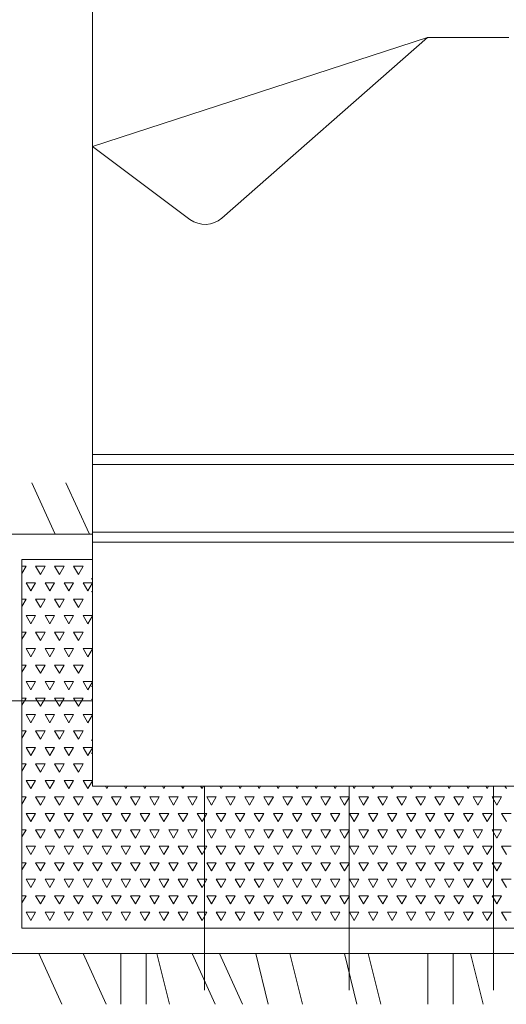
# Model space of a CAD drawing. Units: millimetres. Extents: x 225995 to 227247, y 225507 to 226008.
# Tile 6 of 23: x 226421 to 226461, y 225786 to 225867. Entities that reach past the tile are written whole.
import ezdxf

# ---------------------------------------------------------------- set-up
doc = ezdxf.new("R2010")
doc.units = ezdxf.units.MM
doc.layers.add('A-FLOR-PATT', color=8, linetype='Continuous', lineweight=13)
doc.layers.add('A-FURN', color=9, linetype='Continuous', lineweight=18)

# ---------------------------------------------------------------- blocks, each defined once
blk = doc.blocks.new('A$C6D2A2628')
for p, q in [((0.291, 0.4297), (0.291, 2.4297)), ((0.291, 1.6908), (0.9515, 1.9058)), ((0.9515, 1.9058), (0.5462, 1.5497)), ((0.9515, 1.9058), (1.1116, 1.9058)), ((0.4832, 1.5472), (0.291, 1.6908)), ((0.291, 1.0837), (1.791, 1.0837)), ((0.291, 1.0637), (1.791, 1.0637)), ((0.1716, 1.0278), (0.217, 0.9278)), ((0.2388, 1.0278), (0.2843, 0.9278)), ((0.291, 0.9267), (0.1019, 0.9267)), ((0.291, 0.9307), (1.791, 0.9307)), ((0.291, 0.9107), (1.791, 0.9107)), ((0.291, 0.8767), (0.1519, 0.8767)), ((0.1519, 0.8767), (0.1519, 0.15)), ((0.1519, 0.8494), (0.1601, 0.8636)), ((0.1519, 0.8636), (0.1601, 0.8636)), ((0.1882, 0.8473), (0.1788, 0.8636)), ((0.1788, 0.8636), (0.1976, 0.8636)), ((0.1882, 0.8473), (0.1976, 0.8636)), ((0.2257, 0.8473), (0.2163, 0.8636)), ((0.2163, 0.8636), (0.2351, 0.8636)), ((0.2257, 0.8473), (0.2351, 0.8636)), ((0.2632, 0.8473), (0.2538, 0.8636)), ((0.2538, 0.8636), (0.2726, 0.8636)), ((0.2632, 0.8473), (0.2726, 0.8636)), ((0.291, 0.8376), (0.2893, 0.8393)), ((0.1695, 0.8148), (0.1601, 0.8311)), ((0.1601, 0.8311), (0.1788, 0.8311)), ((0.1695, 0.8148), (0.1788, 0.8311)), ((0.207, 0.8148), (0.1976, 0.8311)), ((0.1976, 0.8311), (0.2163, 0.8311)), ((0.207, 0.8148), (0.2163, 0.8311)), ((0.2445, 0.8148), (0.2351, 0.8311)), ((0.2351, 0.8311), (0.2538, 0.8311)), ((0.2445, 0.8148), (0.2538, 0.8311)), ((0.282, 0.8148), (0.2726, 0.8311)), ((0.2726, 0.8311), (0.291, 0.8311)), ((0.282, 0.8148), (0.291, 0.8305)), ((0.1519, 0.7844), (0.1601, 0.7986)), ((0.1519, 0.7986), (0.1601, 0.7986)), ((0.1882, 0.7824), (0.1788, 0.7986)), ((0.1788, 0.7986), (0.1976, 0.7986)), ((0.1882, 0.7824), (0.1976, 0.7986)), ((0.2257, 0.7824), (0.2163, 0.7986)), ((0.2163, 0.7986), (0.2351, 0.7986)), ((0.2257, 0.7824), (0.2351, 0.7986)), ((0.2632, 0.7824), (0.2538, 0.7986)), ((0.2538, 0.7986), (0.2726, 0.7986)), ((0.2632, 0.7824), (0.2726, 0.7986)), ((0.291, 0.8144), (0.2893, 0.8128)), ((0.1695, 0.7499), (0.1601, 0.7661)), ((0.1601, 0.7661), (0.1788, 0.7661)), ((0.1695, 0.7499), (0.1788, 0.7661)), ((0.207, 0.7499), (0.1976, 0.7661)), ((0.1976, 0.7661), (0.2163, 0.7661)), ((0.207, 0.7499), (0.2163, 0.7661)), ((0.2445, 0.7499), (0.2351, 0.7661)), ((0.2351, 0.7661), (0.2538, 0.7661)), ((0.2445, 0.7499), (0.2538, 0.7661)), ((0.282, 0.7499), (0.2726, 0.7661)), ((0.2726, 0.7661), (0.291, 0.7661)), ((0.282, 0.7499), (0.291, 0.7655)), ((0.1519, 0.7195), (0.1601, 0.7337)), ((0.1519, 0.7337), (0.1601, 0.7337)), ((0.1882, 0.7174), (0.1788, 0.7337)), ((0.1788, 0.7337), (0.1976, 0.7337)), ((0.1882, 0.7174), (0.1976, 0.7337)), ((0.2257, 0.7174), (0.2163, 0.7337)), ((0.2163, 0.7337), (0.2351, 0.7337)), ((0.2257, 0.7174), (0.2351, 0.7337)), ((0.2632, 0.7174), (0.2538, 0.7337)), ((0.2538, 0.7337), (0.2726, 0.7337)), ((0.2632, 0.7174), (0.2726, 0.7337)), ((0.1695, 0.6849), (0.1601, 0.7012)), ((0.1601, 0.7012), (0.1788, 0.7012)), ((0.1695, 0.6849), (0.1788, 0.7012)), ((0.207, 0.6849), (0.1976, 0.7012)), ((0.1976, 0.7012), (0.2163, 0.7012)), ((0.207, 0.6849), (0.2163, 0.7012)), ((0.2445, 0.6849), (0.2351, 0.7012)), ((0.2351, 0.7012), (0.2538, 0.7012)), ((0.2445, 0.6849), (0.2538, 0.7012)), ((0.282, 0.6849), (0.2726, 0.7012)), ((0.2726, 0.7012), (0.291, 0.7012)), ((0.282, 0.6849), (0.291, 0.7006)), ((0.1519, 0.6545), (0.1601, 0.6687)), ((0.1519, 0.6687), (0.1601, 0.6687)), ((0.1882, 0.6525), (0.1788, 0.6687)), ((0.1788, 0.6687), (0.1976, 0.6687)), ((0.1882, 0.6525), (0.1976, 0.6687)), ((0.2257, 0.6525), (0.2163, 0.6687)), ((0.2163, 0.6687), (0.2351, 0.6687)), ((0.2257, 0.6525), (0.2351, 0.6687)), ((0.2632, 0.6525), (0.2538, 0.6687)), ((0.2538, 0.6687), (0.2726, 0.6687)), ((0.2632, 0.6525), (0.2726, 0.6687)), ((0.1695, 0.62), (0.1601, 0.6362)), ((0.1601, 0.6362), (0.1788, 0.6362)), ((0.1695, 0.62), (0.1788, 0.6362)), ((0.207, 0.62), (0.1976, 0.6362)), ((0.1976, 0.6362), (0.2163, 0.6362)), ((0.207, 0.62), (0.2163, 0.6362)), ((0.2445, 0.62), (0.2351, 0.6362)), ((0.2351, 0.6362), (0.2538, 0.6362)), ((0.2445, 0.62), (0.2538, 0.6362)), ((0.282, 0.62), (0.2726, 0.6362)), ((0.2726, 0.6362), (0.291, 0.6362)), ((0.282, 0.62), (0.291, 0.6356)), ((0.291, 0.6255), (0.2893, 0.6271)), ((0.1519, 0.5896), (0.1601, 0.6037)), ((0.1519, 0.6037), (0.1601, 0.6037)), ((0.1882, 0.5875), (0.1788, 0.6037)), ((0.1788, 0.6037), (0.1976, 0.6037)), ((0.1882, 0.5875), (0.1976, 0.6037)), ((0.2257, 0.5875), (0.2163, 0.6037)), ((0.2163, 0.6037), (0.2351, 0.6037)), ((0.2257, 0.5875), (0.2351, 0.6037)), ((0.2632, 0.5875), (0.2538, 0.6037)), ((0.2538, 0.6037), (0.2726, 0.6037)), ((0.2632, 0.5875), (0.2726, 0.6037)), ((0.291, 0.6023), (0.2893, 0.6006)), ((0.1695, 0.555), (0.1601, 0.5713)), ((0.1601, 0.5713), (0.1788, 0.5713)), ((0.1695, 0.555), (0.1788, 0.5713)), ((0.207, 0.555), (0.1976, 0.5713)), ((0.1976, 0.5713), (0.2163, 0.5713)), ((0.207, 0.555), (0.2163, 0.5713)), ((0.2445, 0.555), (0.2351, 0.5713)), ((0.2351, 0.5713), (0.2538, 0.5713)), ((0.2445, 0.555), (0.2538, 0.5713)), ((0.282, 0.555), (0.2726, 0.5713)), ((0.2726, 0.5713), (0.291, 0.5713)), ((0.282, 0.555), (0.291, 0.5707)), ((0.1519, 0.5246), (0.1601, 0.5388)), ((0.1519, 0.5388), (0.1601, 0.5388)), ((0.1882, 0.5226), (0.1788, 0.5388)), ((0.1788, 0.5388), (0.1976, 0.5388)), ((0.1882, 0.5226), (0.1976, 0.5388)), ((0.2257, 0.5226), (0.2163, 0.5388)), ((0.2163, 0.5388), (0.2351, 0.5388)), ((0.2257, 0.5226), (0.2351, 0.5388)), ((0.2632, 0.5226), (0.2538, 0.5388)), ((0.2538, 0.5388), (0.2726, 0.5388)), ((0.2632, 0.5226), (0.2726, 0.5388)), ((0.1695, 0.4901), (0.1601, 0.5063)), ((0.1601, 0.5063), (0.1788, 0.5063)), ((0.1695, 0.4901), (0.1788, 0.5063)), ((0.207, 0.4901), (0.1976, 0.5063)), ((0.1976, 0.5063), (0.2163, 0.5063)), ((0.207, 0.4901), (0.2163, 0.5063)), ((0.2445, 0.4901), (0.2351, 0.5063)), ((0.2351, 0.5063), (0.2538, 0.5063)), ((0.2445, 0.4901), (0.2538, 0.5063)), ((0.282, 0.4901), (0.2726, 0.5063)), ((0.2726, 0.5063), (0.291, 0.5063)), ((0.282, 0.4901), (0.291, 0.5057)), ((0.291, 0.5194), (0.2893, 0.5211)), ((0.291, 0.4962), (0.2893, 0.4946)), ((0.1519, 0.4597), (0.1601, 0.4738)), ((0.1519, 0.4738), (0.1601, 0.4738)), ((0.1882, 0.4576), (0.1788, 0.4738)), ((0.1788, 0.4738), (0.1976, 0.4738)), ((0.1882, 0.4576), (0.1976, 0.4738)), ((0.2257, 0.4576), (0.2163, 0.4738)), ((0.2163, 0.4738), (0.2351, 0.4738)), ((0.2257, 0.4576), (0.2351, 0.4738)), ((0.2632, 0.4576), (0.2538, 0.4738)), ((0.2538, 0.4738), (0.2726, 0.4738)), ((0.2632, 0.4576), (0.2726, 0.4738)), ((0.1695, 0.4251), (0.1601, 0.4414)), ((0.1601, 0.4414), (0.1788, 0.4414)), ((0.1695, 0.4251), (0.1788, 0.4414)), ((0.207, 0.4251), (0.1976, 0.4414)), ((0.1976, 0.4414), (0.2163, 0.4414)), ((0.207, 0.4251), (0.2163, 0.4414)), ((0.2445, 0.4251), (0.2351, 0.4414)), ((0.2351, 0.4414), (0.2538, 0.4414)), ((0.2445, 0.4251), (0.2538, 0.4414)), ((0.282, 0.4251), (0.2726, 0.4414)), ((0.2726, 0.4414), (0.291, 0.4414)), ((0.282, 0.4251), (0.291, 0.4408)), ((1.791, 0.4297), (0.291, 0.4297)), ((0.3195, 0.4251), (0.3168, 0.4297)), ((0.3195, 0.4251), (0.3221, 0.4297)), ((0.357, 0.4251), (0.3543, 0.4297)), ((0.357, 0.4251), (0.3596, 0.4297)), ((0.3945, 0.4251), (0.3918, 0.4297)), ((0.3945, 0.4251), (0.3971, 0.4297)), ((0.432, 0.4251), (0.4293, 0.4297)), ((0.432, 0.4251), (0.4346, 0.4297)), ((0.4695, 0.4251), (0.4668, 0.4297)), ((0.4695, 0.4251), (0.4721, 0.4297)), ((0.507, 0.4251), (0.5043, 0.4297)), ((0.507, 0.4251), (0.5096, 0.4297)), ((0.5445, 0.4251), (0.5418, 0.4297)), ((0.5445, 0.4251), (0.5471, 0.4297)), ((0.582, 0.4251), (0.5793, 0.4297)), ((0.582, 0.4251), (0.5846, 0.4297)), ((0.6195, 0.4251), (0.6168, 0.4297)), ((0.6195, 0.4251), (0.6221, 0.4297)), ((0.657, 0.4251), (0.6543, 0.4297)), ((0.657, 0.4251), (0.6596, 0.4297)), ((0.6945, 0.4251), (0.6918, 0.4297)), ((0.6945, 0.4251), (0.6971, 0.4297)), ((0.732, 0.4251), (0.7293, 0.4297)), ((0.732, 0.4251), (0.7346, 0.4297)), ((0.7695, 0.4251), (0.7668, 0.4297)), ((0.7695, 0.4251), (0.7721, 0.4297)), ((0.807, 0.4251), (0.8043, 0.4297)), ((0.807, 0.4251), (0.8096, 0.4297)), ((0.8445, 0.4251), (0.8418, 0.4297)), ((0.8445, 0.4251), (0.8471, 0.4297)), ((0.882, 0.4251), (0.8793, 0.4297)), ((0.882, 0.4251), (0.8846, 0.4297)), ((0.9195, 0.4251), (0.9168, 0.4297)), ((0.9195, 0.4251), (0.9221, 0.4297)), ((0.957, 0.4251), (0.9543, 0.4297)), ((0.957, 0.4251), (0.9596, 0.4297)), ((0.9945, 0.4251), (0.9918, 0.4297)), ((0.9945, 0.4251), (0.9971, 0.4297)), ((1.032, 0.4251), (1.0293, 0.4297)), ((1.032, 0.4251), (1.0346, 0.4297)), ((1.0695, 0.4251), (1.0668, 0.4297)), ((1.0695, 0.4251), (1.0721, 0.4297)), ((1.107, 0.4251), (1.1043, 0.4297)), ((0.1519, 0.3947), (0.1601, 0.4089)), ((0.1519, 0.4089), (0.1601, 0.4089)), ((0.1882, 0.3927), (0.1788, 0.4089)), ((0.1788, 0.4089), (0.1976, 0.4089)), ((0.1882, 0.3927), (0.1976, 0.4089)), ((0.2257, 0.3927), (0.2163, 0.4089)), ((0.2163, 0.4089), (0.2351, 0.4089)), ((0.2257, 0.3927), (0.2351, 0.4089)), ((0.2632, 0.3927), (0.2538, 0.4089)), ((0.2538, 0.4089), (0.2726, 0.4089)), ((0.2632, 0.3927), (0.2726, 0.4089)), ((0.3007, 0.3927), (0.2913, 0.4089)), ((0.2913, 0.4089), (0.3101, 0.4089)), ((0.3007, 0.3927), (0.3101, 0.4089)), ((0.3382, 0.3927), (0.3288, 0.4089)), ((0.3288, 0.4089), (0.3476, 0.4089)), ((0.3382, 0.3927), (0.3476, 0.4089)), ((0.3757, 0.3927), (0.3663, 0.4089)), ((0.3663, 0.4089), (0.3851, 0.4089)), ((0.3757, 0.3927), (0.3851, 0.4089)), ((0.4132, 0.3927), (0.4038, 0.4089)), ((0.4038, 0.4089), (0.4226, 0.4089)), ((0.4132, 0.3927), (0.4226, 0.4089)), ((0.4507, 0.3927), (0.4413, 0.4089)), ((0.4413, 0.4089), (0.4601, 0.4089)), ((0.4507, 0.3927), (0.4601, 0.4089)), ((0.4882, 0.3927), (0.4788, 0.4089)), ((0.4788, 0.4089), (0.4976, 0.4089)), ((0.4882, 0.3927), (0.4976, 0.4089)), ((0.5257, 0.3927), (0.5163, 0.4089)), ((0.5163, 0.4089), (0.5351, 0.4089)), ((0.5257, 0.3927), (0.5351, 0.4089)), ((0.5632, 0.3927), (0.5538, 0.4089)), ((0.5538, 0.4089), (0.5726, 0.4089)), ((0.5632, 0.3927), (0.5726, 0.4089)), ((0.6007, 0.3927), (0.5913, 0.4089)), ((0.5913, 0.4089), (0.6101, 0.4089)), ((0.6007, 0.3927), (0.6101, 0.4089)), ((0.6382, 0.3927), (0.6288, 0.4089)), ((0.6288, 0.4089), (0.6476, 0.4089)), ((0.6382, 0.3927), (0.6476, 0.4089)), ((0.6757, 0.3927), (0.6663, 0.4089)), ((0.6663, 0.4089), (0.6851, 0.4089)), ((0.6757, 0.3927), (0.6851, 0.4089)), ((0.7132, 0.3927), (0.7038, 0.4089)), ((0.7038, 0.4089), (0.7226, 0.4089)), ((0.7132, 0.3927), (0.7226, 0.4089)), ((0.7507, 0.3927), (0.7413, 0.4089)), ((0.7413, 0.4089), (0.7601, 0.4089)), ((0.7507, 0.3927), (0.7601, 0.4089)), ((0.7882, 0.3927), (0.7788, 0.4089)), ((0.7788, 0.4089), (0.7976, 0.4089)), ((0.7882, 0.3927), (0.7976, 0.4089)), ((0.8257, 0.3927), (0.8163, 0.4089)), ((0.8163, 0.4089), (0.8351, 0.4089)), ((0.8257, 0.3927), (0.8351, 0.4089)), ((0.8632, 0.3927), (0.8538, 0.4089)), ((0.8538, 0.4089), (0.8726, 0.4089)), ((0.8632, 0.3927), (0.8726, 0.4089)), ((0.9007, 0.3927), (0.8913, 0.4089)), ((0.8913, 0.4089), (0.9101, 0.4089)), ((0.9007, 0.3927), (0.9101, 0.4089)), ((0.9382, 0.3927), (0.9288, 0.4089)), ((0.9288, 0.4089), (0.9476, 0.4089)), ((0.9382, 0.3927), (0.9476, 0.4089)), ((0.9757, 0.3927), (0.9663, 0.4089)), ((0.9663, 0.4089), (0.9851, 0.4089)), ((0.9757, 0.3927), (0.9851, 0.4089)), ((1.0132, 0.3927), (1.0038, 0.4089)), ((1.0038, 0.4089), (1.0226, 0.4089)), ((1.0132, 0.3927), (1.0226, 0.4089)), ((1.0507, 0.3927), (1.0413, 0.4089)), ((1.0413, 0.4089), (1.0601, 0.4089)), ((1.0507, 0.3927), (1.0601, 0.4089)), ((1.0882, 0.3927), (1.0788, 0.4089)), ((1.0788, 0.4089), (1.0976, 0.4089)), ((1.0882, 0.3927), (1.0976, 0.4089)), ((0.1695, 0.3602), (0.1601, 0.3764)), ((0.1601, 0.3764), (0.1788, 0.3764)), ((0.1695, 0.3602), (0.1788, 0.3764)), ((0.207, 0.3602), (0.1976, 0.3764)), ((0.1976, 0.3764), (0.2163, 0.3764)), ((0.207, 0.3602), (0.2163, 0.3764)), ((0.2445, 0.3602), (0.2351, 0.3764)), ((0.2351, 0.3764), (0.2538, 0.3764)), ((0.2445, 0.3602), (0.2538, 0.3764)), ((0.282, 0.3602), (0.2726, 0.3764)), ((0.2726, 0.3764), (0.2913, 0.3764)), ((0.282, 0.3602), (0.2913, 0.3764)), ((0.3195, 0.3602), (0.3101, 0.3764)), ((0.3101, 0.3764), (0.3288, 0.3764)), ((0.3195, 0.3602), (0.3288, 0.3764)), ((0.357, 0.3602), (0.3476, 0.3764)), ((0.3476, 0.3764), (0.3663, 0.3764)), ((0.357, 0.3602), (0.3663, 0.3764)), ((0.3945, 0.3602), (0.3851, 0.3764)), ((0.3851, 0.3764), (0.4038, 0.3764)), ((0.3945, 0.3602), (0.4038, 0.3764)), ((0.432, 0.3602), (0.4226, 0.3764)), ((0.4226, 0.3764), (0.4413, 0.3764)), ((0.432, 0.3602), (0.4413, 0.3764)), ((0.4695, 0.3602), (0.4601, 0.3764)), ((0.4601, 0.3764), (0.4788, 0.3764)), ((0.4695, 0.3602), (0.4788, 0.3764)), ((0.507, 0.3602), (0.4976, 0.3764)), ((0.4976, 0.3764), (0.5163, 0.3764)), ((0.507, 0.3602), (0.5163, 0.3764)), ((0.5445, 0.3602), (0.5351, 0.3764)), ((0.5351, 0.3764), (0.5538, 0.3764)), ((0.5445, 0.3602), (0.5538, 0.3764)), ((0.582, 0.3602), (0.5726, 0.3764)), ((0.5726, 0.3764), (0.5913, 0.3764)), ((0.582, 0.3602), (0.5913, 0.3764)), ((0.6195, 0.3602), (0.6101, 0.3764)), ((0.6101, 0.3764), (0.6288, 0.3764)), ((0.6195, 0.3602), (0.6288, 0.3764)), ((0.657, 0.3602), (0.6476, 0.3764)), ((0.6476, 0.3764), (0.6663, 0.3764)), ((0.657, 0.3602), (0.6663, 0.3764)), ((0.6945, 0.3602), (0.6851, 0.3764)), ((0.6851, 0.3764), (0.7038, 0.3764)), ((0.6945, 0.3602), (0.7038, 0.3764)), ((0.732, 0.3602), (0.7226, 0.3764)), ((0.7226, 0.3764), (0.7413, 0.3764)), ((0.732, 0.3602), (0.7413, 0.3764)), ((0.7695, 0.3602), (0.7601, 0.3764)), ((0.7601, 0.3764), (0.7788, 0.3764)), ((0.7695, 0.3602), (0.7788, 0.3764)), ((0.807, 0.3602), (0.7976, 0.3764)), ((0.7976, 0.3764), (0.8163, 0.3764)), ((0.807, 0.3602), (0.8163, 0.3764)), ((0.8445, 0.3602), (0.8351, 0.3764)), ((0.8351, 0.3764), (0.8538, 0.3764)), ((0.8445, 0.3602), (0.8538, 0.3764)), ((0.882, 0.3602), (0.8726, 0.3764)), ((0.8726, 0.3764), (0.8913, 0.3764)), ((0.882, 0.3602), (0.8913, 0.3764)), ((0.9195, 0.3602), (0.9101, 0.3764)), ((0.9101, 0.3764), (0.9288, 0.3764)), ((0.9195, 0.3602), (0.9288, 0.3764)), ((0.957, 0.3602), (0.9476, 0.3764)), ((0.9476, 0.3764), (0.9663, 0.3764)), ((0.957, 0.3602), (0.9663, 0.3764)), ((0.9945, 0.3602), (0.9851, 0.3764)), ((0.9851, 0.3764), (1.0038, 0.3764)), ((0.9945, 0.3602), (1.0038, 0.3764)), ((1.032, 0.3602), (1.0226, 0.3764)), ((1.0226, 0.3764), (1.0413, 0.3764)), ((1.032, 0.3602), (1.0413, 0.3764)), ((1.0695, 0.3602), (1.0601, 0.3764)), ((1.0601, 0.3764), (1.0788, 0.3764)), ((1.0695, 0.3602), (1.0788, 0.3764)), ((1.107, 0.3602), (1.0976, 0.3764)), ((1.0976, 0.3764), (1.1163, 0.3764)), ((0.1519, 0.3298), (0.1601, 0.3439)), ((0.1519, 0.3439), (0.1601, 0.3439)), ((0.1882, 0.3277), (0.1788, 0.3439)), ((0.1788, 0.3439), (0.1976, 0.3439)), ((0.1882, 0.3277), (0.1976, 0.3439)), ((0.2257, 0.3277), (0.2163, 0.3439)), ((0.2163, 0.3439), (0.2351, 0.3439)), ((0.2257, 0.3277), (0.2351, 0.3439)), ((0.2632, 0.3277), (0.2538, 0.3439)), ((0.2538, 0.3439), (0.2726, 0.3439)), ((0.2632, 0.3277), (0.2726, 0.3439)), ((0.3007, 0.3277), (0.2913, 0.3439)), ((0.2913, 0.3439), (0.3101, 0.3439)), ((0.3007, 0.3277), (0.3101, 0.3439)), ((0.3382, 0.3277), (0.3288, 0.3439)), ((0.3288, 0.3439), (0.3476, 0.3439)), ((0.3382, 0.3277), (0.3476, 0.3439)), ((0.3757, 0.3277), (0.3663, 0.3439)), ((0.3663, 0.3439), (0.3851, 0.3439)), ((0.3757, 0.3277), (0.3851, 0.3439)), ((0.4132, 0.3277), (0.4038, 0.3439)), ((0.4038, 0.3439), (0.4226, 0.3439)), ((0.4132, 0.3277), (0.4226, 0.3439)), ((0.4507, 0.3277), (0.4413, 0.3439)), ((0.4413, 0.3439), (0.4601, 0.3439)), ((0.4507, 0.3277), (0.4601, 0.3439)), ((0.4882, 0.3277), (0.4788, 0.3439)), ((0.4788, 0.3439), (0.4976, 0.3439)), ((0.4882, 0.3277), (0.4976, 0.3439)), ((0.5257, 0.3277), (0.5163, 0.3439)), ((0.5163, 0.3439), (0.5351, 0.3439)), ((0.5257, 0.3277), (0.5351, 0.3439)), ((0.5632, 0.3277), (0.5538, 0.3439)), ((0.5538, 0.3439), (0.5726, 0.3439)), ((0.5632, 0.3277), (0.5726, 0.3439)), ((0.6007, 0.3277), (0.5913, 0.3439)), ((0.5913, 0.3439), (0.6101, 0.3439)), ((0.6007, 0.3277), (0.6101, 0.3439)), ((0.6382, 0.3277), (0.6288, 0.3439)), ((0.6288, 0.3439), (0.6476, 0.3439)), ((0.6382, 0.3277), (0.6476, 0.3439)), ((0.6757, 0.3277), (0.6663, 0.3439)), ((0.6663, 0.3439), (0.6851, 0.3439)), ((0.6757, 0.3277), (0.6851, 0.3439)), ((0.7132, 0.3277), (0.7038, 0.3439)), ((0.7038, 0.3439), (0.7226, 0.3439)), ((0.7132, 0.3277), (0.7226, 0.3439)), ((0.7507, 0.3277), (0.7413, 0.3439)), ((0.7413, 0.3439), (0.7601, 0.3439)), ((0.7507, 0.3277), (0.7601, 0.3439)), ((0.7882, 0.3277), (0.7788, 0.3439)), ((0.7788, 0.3439), (0.7976, 0.3439)), ((0.7882, 0.3277), (0.7976, 0.3439)), ((0.8257, 0.3277), (0.8163, 0.3439)), ((0.8163, 0.3439), (0.8351, 0.3439)), ((0.8257, 0.3277), (0.8351, 0.3439)), ((0.8632, 0.3277), (0.8538, 0.3439)), ((0.8538, 0.3439), (0.8726, 0.3439)), ((0.8632, 0.3277), (0.8726, 0.3439)), ((0.9007, 0.3277), (0.8913, 0.3439)), ((0.8913, 0.3439), (0.9101, 0.3439)), ((0.9007, 0.3277), (0.9101, 0.3439)), ((0.9382, 0.3277), (0.9288, 0.3439)), ((0.9288, 0.3439), (0.9476, 0.3439)), ((0.9382, 0.3277), (0.9476, 0.3439)), ((0.9757, 0.3277), (0.9663, 0.3439)), ((0.9663, 0.3439), (0.9851, 0.3439)), ((0.9757, 0.3277), (0.9851, 0.3439)), ((1.0132, 0.3277), (1.0038, 0.3439)), ((1.0038, 0.3439), (1.0226, 0.3439)), ((1.0132, 0.3277), (1.0226, 0.3439)), ((1.0507, 0.3277), (1.0413, 0.3439)), ((1.0413, 0.3439), (1.0601, 0.3439)), ((1.0507, 0.3277), (1.0601, 0.3439)), ((1.0882, 0.3277), (1.0788, 0.3439)), ((1.0788, 0.3439), (1.0976, 0.3439)), ((1.0882, 0.3277), (1.0976, 0.3439)), ((0.1695, 0.2952), (0.1601, 0.3115)), ((0.1601, 0.3115), (0.1788, 0.3115)), ((0.1695, 0.2952), (0.1788, 0.3115)), ((0.207, 0.2952), (0.1976, 0.3115)), ((0.1976, 0.3115), (0.2163, 0.3115)), ((0.207, 0.2952), (0.2163, 0.3115)), ((0.2445, 0.2952), (0.2351, 0.3115)), ((0.2351, 0.3115), (0.2538, 0.3115)), ((0.2445, 0.2952), (0.2538, 0.3115)), ((0.282, 0.2952), (0.2726, 0.3115)), ((0.2726, 0.3115), (0.2913, 0.3115)), ((0.282, 0.2952), (0.2913, 0.3115)), ((0.3195, 0.2952), (0.3101, 0.3115)), ((0.3101, 0.3115), (0.3288, 0.3115)), ((0.3195, 0.2952), (0.3288, 0.3115)), ((0.357, 0.2952), (0.3476, 0.3115)), ((0.3476, 0.3115), (0.3663, 0.3115)), ((0.357, 0.2952), (0.3663, 0.3115)), ((0.3945, 0.2952), (0.3851, 0.3115)), ((0.3851, 0.3115), (0.4038, 0.3115)), ((0.3945, 0.2952), (0.4038, 0.3115)), ((0.432, 0.2952), (0.4226, 0.3115)), ((0.4226, 0.3115), (0.4413, 0.3115)), ((0.432, 0.2952), (0.4413, 0.3115)), ((0.4695, 0.2952), (0.4601, 0.3115)), ((0.4601, 0.3115), (0.4788, 0.3115)), ((0.4695, 0.2952), (0.4788, 0.3115)), ((0.507, 0.2952), (0.4976, 0.3115)), ((0.4976, 0.3115), (0.5163, 0.3115)), ((0.507, 0.2952), (0.5163, 0.3115)), ((0.5445, 0.2952), (0.5351, 0.3115)), ((0.5351, 0.3115), (0.5538, 0.3115)), ((0.5445, 0.2952), (0.5538, 0.3115)), ((0.582, 0.2952), (0.5726, 0.3115)), ((0.5726, 0.3115), (0.5913, 0.3115)), ((0.582, 0.2952), (0.5913, 0.3115)), ((0.6195, 0.2952), (0.6101, 0.3115)), ((0.6101, 0.3115), (0.6288, 0.3115)), ((0.6195, 0.2952), (0.6288, 0.3115)), ((0.657, 0.2952), (0.6476, 0.3115)), ((0.6476, 0.3115), (0.6663, 0.3115)), ((0.657, 0.2952), (0.6663, 0.3115)), ((0.6945, 0.2952), (0.6851, 0.3115)), ((0.6851, 0.3115), (0.7038, 0.3115)), ((0.6945, 0.2952), (0.7038, 0.3115)), ((0.732, 0.2952), (0.7226, 0.3115)), ((0.7226, 0.3115), (0.7413, 0.3115)), ((0.732, 0.2952), (0.7413, 0.3115)), ((0.7695, 0.2952), (0.7601, 0.3115)), ((0.7601, 0.3115), (0.7788, 0.3115)), ((0.7695, 0.2952), (0.7788, 0.3115)), ((0.807, 0.2952), (0.7976, 0.3115)), ((0.7976, 0.3115), (0.8163, 0.3115)), ((0.807, 0.2952), (0.8163, 0.3115)), ((0.8445, 0.2952), (0.8351, 0.3115)), ((0.8351, 0.3115), (0.8538, 0.3115)), ((0.8445, 0.2952), (0.8538, 0.3115)), ((0.882, 0.2952), (0.8726, 0.3115)), ((0.8726, 0.3115), (0.8913, 0.3115)), ((0.882, 0.2952), (0.8913, 0.3115)), ((0.9195, 0.2952), (0.9101, 0.3115)), ((0.9101, 0.3115), (0.9288, 0.3115)), ((0.9195, 0.2952), (0.9288, 0.3115)), ((0.957, 0.2952), (0.9476, 0.3115)), ((0.9476, 0.3115), (0.9663, 0.3115)), ((0.957, 0.2952), (0.9663, 0.3115)), ((0.9945, 0.2952), (0.9851, 0.3115)), ((0.9851, 0.3115), (1.0038, 0.3115)), ((0.9945, 0.2952), (1.0038, 0.3115)), ((1.032, 0.2952), (1.0226, 0.3115)), ((1.0226, 0.3115), (1.0413, 0.3115)), ((1.032, 0.2952), (1.0413, 0.3115)), ((1.0695, 0.2952), (1.0601, 0.3115)), ((1.0601, 0.3115), (1.0788, 0.3115)), ((1.0695, 0.2952), (1.0788, 0.3115)), ((1.107, 0.2952), (1.0976, 0.3115)), ((1.0976, 0.3115), (1.1163, 0.3115)), ((0.1519, 0.2648), (0.1601, 0.279)), ((0.1519, 0.279), (0.1601, 0.279)), ((0.1882, 0.2628), (0.1788, 0.279)), ((0.1788, 0.279), (0.1976, 0.279)), ((0.1882, 0.2628), (0.1976, 0.279)), ((0.2257, 0.2628), (0.2163, 0.279)), ((0.2163, 0.279), (0.2351, 0.279)), ((0.2257, 0.2628), (0.2351, 0.279)), ((0.2632, 0.2628), (0.2538, 0.279)), ((0.2538, 0.279), (0.2726, 0.279)), ((0.2632, 0.2628), (0.2726, 0.279)), ((0.3007, 0.2628), (0.2913, 0.279)), ((0.2913, 0.279), (0.3101, 0.279)), ((0.3007, 0.2628), (0.3101, 0.279)), ((0.3382, 0.2628), (0.3288, 0.279)), ((0.3288, 0.279), (0.3476, 0.279)), ((0.3382, 0.2628), (0.3476, 0.279)), ((0.3757, 0.2628), (0.3663, 0.279)), ((0.3663, 0.279), (0.3851, 0.279)), ((0.3757, 0.2628), (0.3851, 0.279)), ((0.4132, 0.2628), (0.4038, 0.279)), ((0.4038, 0.279), (0.4226, 0.279)), ((0.4132, 0.2628), (0.4226, 0.279)), ((0.4507, 0.2628), (0.4413, 0.279)), ((0.4413, 0.279), (0.4601, 0.279)), ((0.4507, 0.2628), (0.4601, 0.279)), ((0.4882, 0.2628), (0.4788, 0.279)), ((0.4788, 0.279), (0.4976, 0.279)), ((0.4882, 0.2628), (0.4976, 0.279)), ((0.5257, 0.2628), (0.5163, 0.279)), ((0.5163, 0.279), (0.5351, 0.279)), ((0.5257, 0.2628), (0.5351, 0.279)), ((0.5632, 0.2628), (0.5538, 0.279)), ((0.5538, 0.279), (0.5726, 0.279)), ((0.5632, 0.2628), (0.5726, 0.279)), ((0.6007, 0.2628), (0.5913, 0.279)), ((0.5913, 0.279), (0.6101, 0.279)), ((0.6007, 0.2628), (0.6101, 0.279)), ((0.6382, 0.2628), (0.6288, 0.279)), ((0.6288, 0.279), (0.6476, 0.279)), ((0.6382, 0.2628), (0.6476, 0.279)), ((0.6757, 0.2628), (0.6663, 0.279)), ((0.6663, 0.279), (0.6851, 0.279)), ((0.6757, 0.2628), (0.6851, 0.279)), ((0.7132, 0.2628), (0.7038, 0.279)), ((0.7038, 0.279), (0.7226, 0.279)), ((0.7132, 0.2628), (0.7226, 0.279)), ((0.7507, 0.2628), (0.7413, 0.279)), ((0.7413, 0.279), (0.7601, 0.279)), ((0.7507, 0.2628), (0.7601, 0.279)), ((0.7882, 0.2628), (0.7788, 0.279)), ((0.7788, 0.279), (0.7976, 0.279)), ((0.7882, 0.2628), (0.7976, 0.279)), ((0.8257, 0.2628), (0.8163, 0.279)), ((0.8163, 0.279), (0.8351, 0.279)), ((0.8257, 0.2628), (0.8351, 0.279)), ((0.8632, 0.2628), (0.8538, 0.279)), ((0.8538, 0.279), (0.8726, 0.279)), ((0.8632, 0.2628), (0.8726, 0.279)), ((0.9007, 0.2628), (0.8913, 0.279)), ((0.8913, 0.279), (0.9101, 0.279)), ((0.9007, 0.2628), (0.9101, 0.279)), ((0.9382, 0.2628), (0.9288, 0.279)), ((0.9288, 0.279), (0.9476, 0.279)), ((0.9382, 0.2628), (0.9476, 0.279)), ((0.9757, 0.2628), (0.9663, 0.279)), ((0.9663, 0.279), (0.9851, 0.279)), ((0.9757, 0.2628), (0.9851, 0.279)), ((1.0132, 0.2628), (1.0038, 0.279)), ((1.0038, 0.279), (1.0226, 0.279)), ((1.0132, 0.2628), (1.0226, 0.279)), ((1.0507, 0.2628), (1.0413, 0.279)), ((1.0413, 0.279), (1.0601, 0.279)), ((1.0507, 0.2628), (1.0601, 0.279)), ((1.0882, 0.2628), (1.0788, 0.279)), ((1.0788, 0.279), (1.0976, 0.279)), ((1.0882, 0.2628), (1.0976, 0.279)), ((0.1695, 0.2303), (0.1601, 0.2465)), ((0.1601, 0.2465), (0.1788, 0.2465)), ((0.1695, 0.2303), (0.1788, 0.2465)), ((0.207, 0.2303), (0.1976, 0.2465)), ((0.1976, 0.2465), (0.2163, 0.2465)), ((0.207, 0.2303), (0.2163, 0.2465)), ((0.2445, 0.2303), (0.2351, 0.2465)), ((0.2351, 0.2465), (0.2538, 0.2465)), ((0.2445, 0.2303), (0.2538, 0.2465)), ((0.282, 0.2303), (0.2726, 0.2465)), ((0.2726, 0.2465), (0.2913, 0.2465)), ((0.282, 0.2303), (0.2913, 0.2465)), ((0.3195, 0.2303), (0.3101, 0.2465)), ((0.3101, 0.2465), (0.3288, 0.2465)), ((0.3195, 0.2303), (0.3288, 0.2465)), ((0.357, 0.2303), (0.3476, 0.2465)), ((0.3476, 0.2465), (0.3663, 0.2465)), ((0.357, 0.2303), (0.3663, 0.2465)), ((0.3945, 0.2303), (0.3851, 0.2465)), ((0.3851, 0.2465), (0.4038, 0.2465)), ((0.3945, 0.2303), (0.4038, 0.2465)), ((0.432, 0.2303), (0.4226, 0.2465)), ((0.4226, 0.2465), (0.4413, 0.2465)), ((0.432, 0.2303), (0.4413, 0.2465)), ((0.4695, 0.2303), (0.4601, 0.2465)), ((0.4601, 0.2465), (0.4788, 0.2465)), ((0.4695, 0.2303), (0.4788, 0.2465)), ((0.507, 0.2303), (0.4976, 0.2465)), ((0.4976, 0.2465), (0.5163, 0.2465)), ((0.507, 0.2303), (0.5163, 0.2465)), ((0.5445, 0.2303), (0.5351, 0.2465)), ((0.5351, 0.2465), (0.5538, 0.2465)), ((0.5445, 0.2303), (0.5538, 0.2465)), ((0.582, 0.2303), (0.5726, 0.2465)), ((0.5726, 0.2465), (0.5913, 0.2465)), ((0.582, 0.2303), (0.5913, 0.2465)), ((0.6195, 0.2303), (0.6101, 0.2465)), ((0.6101, 0.2465), (0.6288, 0.2465)), ((0.6195, 0.2303), (0.6288, 0.2465)), ((0.657, 0.2303), (0.6476, 0.2465)), ((0.6476, 0.2465), (0.6663, 0.2465)), ((0.657, 0.2303), (0.6663, 0.2465)), ((0.6945, 0.2303), (0.6851, 0.2465)), ((0.6851, 0.2465), (0.7038, 0.2465)), ((0.6945, 0.2303), (0.7038, 0.2465)), ((0.732, 0.2303), (0.7226, 0.2465)), ((0.7226, 0.2465), (0.7413, 0.2465)), ((0.732, 0.2303), (0.7413, 0.2465)), ((0.7695, 0.2303), (0.7601, 0.2465)), ((0.7601, 0.2465), (0.7788, 0.2465)), ((0.7695, 0.2303), (0.7788, 0.2465)), ((0.807, 0.2303), (0.7976, 0.2465)), ((0.7976, 0.2465), (0.8163, 0.2465)), ((0.807, 0.2303), (0.8163, 0.2465)), ((0.8445, 0.2303), (0.8351, 0.2465)), ((0.8351, 0.2465), (0.8538, 0.2465)), ((0.8445, 0.2303), (0.8538, 0.2465)), ((0.882, 0.2303), (0.8726, 0.2465)), ((0.8726, 0.2465), (0.8913, 0.2465)), ((0.882, 0.2303), (0.8913, 0.2465)), ((0.9195, 0.2303), (0.9101, 0.2465)), ((0.9101, 0.2465), (0.9288, 0.2465)), ((0.9195, 0.2303), (0.9288, 0.2465)), ((0.957, 0.2303), (0.9476, 0.2465)), ((0.9476, 0.2465), (0.9663, 0.2465)), ((0.957, 0.2303), (0.9663, 0.2465)), ((0.9945, 0.2303), (0.9851, 0.2465)), ((0.9851, 0.2465), (1.0038, 0.2465)), ((0.9945, 0.2303), (1.0038, 0.2465)), ((1.032, 0.2303), (1.0226, 0.2465)), ((1.0226, 0.2465), (1.0413, 0.2465)), ((1.032, 0.2303), (1.0413, 0.2465)), ((1.0695, 0.2303), (1.0601, 0.2465)), ((1.0601, 0.2465), (1.0788, 0.2465)), ((1.0695, 0.2303), (1.0788, 0.2465)), ((1.107, 0.2303), (1.0976, 0.2465)), ((1.0976, 0.2465), (1.1163, 0.2465)), ((0.1519, 0.1999), (0.1601, 0.214)), ((0.1519, 0.214), (0.1601, 0.214)), ((0.1882, 0.1978), (0.1788, 0.214)), ((0.1788, 0.214), (0.1976, 0.214)), ((0.1882, 0.1978), (0.1976, 0.214)), ((0.2257, 0.1978), (0.2163, 0.214)), ((0.2163, 0.214), (0.2351, 0.214)), ((0.2257, 0.1978), (0.2351, 0.214)), ((0.2632, 0.1978), (0.2538, 0.214)), ((0.2538, 0.214), (0.2726, 0.214)), ((0.2632, 0.1978), (0.2726, 0.214)), ((0.3007, 0.1978), (0.2913, 0.214)), ((0.2913, 0.214), (0.3101, 0.214)), ((0.3007, 0.1978), (0.3101, 0.214)), ((0.3382, 0.1978), (0.3288, 0.214)), ((0.3288, 0.214), (0.3476, 0.214)), ((0.3382, 0.1978), (0.3476, 0.214)), ((0.3757, 0.1978), (0.3663, 0.214)), ((0.3663, 0.214), (0.3851, 0.214)), ((0.3757, 0.1978), (0.3851, 0.214)), ((0.4132, 0.1978), (0.4038, 0.214)), ((0.4038, 0.214), (0.4226, 0.214)), ((0.4132, 0.1978), (0.4226, 0.214)), ((0.4507, 0.1978), (0.4413, 0.214)), ((0.4413, 0.214), (0.4601, 0.214)), ((0.4507, 0.1978), (0.4601, 0.214)), ((0.4882, 0.1978), (0.4788, 0.214)), ((0.4788, 0.214), (0.4976, 0.214)), ((0.4882, 0.1978), (0.4976, 0.214)), ((0.5257, 0.1978), (0.5163, 0.214)), ((0.5163, 0.214), (0.5351, 0.214)), ((0.5257, 0.1978), (0.5351, 0.214)), ((0.5632, 0.1978), (0.5538, 0.214)), ((0.5538, 0.214), (0.5726, 0.214)), ((0.5632, 0.1978), (0.5726, 0.214)), ((0.6007, 0.1978), (0.5913, 0.214)), ((0.5913, 0.214), (0.6101, 0.214)), ((0.6007, 0.1978), (0.6101, 0.214)), ((0.6382, 0.1978), (0.6288, 0.214)), ((0.6288, 0.214), (0.6476, 0.214)), ((0.6382, 0.1978), (0.6476, 0.214)), ((0.6757, 0.1978), (0.6663, 0.214)), ((0.6663, 0.214), (0.6851, 0.214)), ((0.6757, 0.1978), (0.6851, 0.214)), ((0.7132, 0.1978), (0.7038, 0.214)), ((0.7038, 0.214), (0.7226, 0.214)), ((0.7132, 0.1978), (0.7226, 0.214)), ((0.7507, 0.1978), (0.7413, 0.214)), ((0.7413, 0.214), (0.7601, 0.214)), ((0.7507, 0.1978), (0.7601, 0.214)), ((0.7882, 0.1978), (0.7788, 0.214)), ((0.7788, 0.214), (0.7976, 0.214)), ((0.7882, 0.1978), (0.7976, 0.214)), ((0.8257, 0.1978), (0.8163, 0.214)), ((0.8163, 0.214), (0.8351, 0.214)), ((0.8257, 0.1978), (0.8351, 0.214)), ((0.8632, 0.1978), (0.8538, 0.214)), ((0.8538, 0.214), (0.8726, 0.214)), ((0.8632, 0.1978), (0.8726, 0.214)), ((0.9007, 0.1978), (0.8913, 0.214)), ((0.8913, 0.214), (0.9101, 0.214)), ((0.9007, 0.1978), (0.9101, 0.214)), ((0.9382, 0.1978), (0.9288, 0.214)), ((0.9288, 0.214), (0.9476, 0.214)), ((0.9382, 0.1978), (0.9476, 0.214)), ((0.9757, 0.1978), (0.9663, 0.214)), ((0.9663, 0.214), (0.9851, 0.214)), ((0.9757, 0.1978), (0.9851, 0.214)), ((1.0132, 0.1978), (1.0038, 0.214)), ((1.0038, 0.214), (1.0226, 0.214)), ((1.0132, 0.1978), (1.0226, 0.214)), ((1.0507, 0.1978), (1.0413, 0.214)), ((1.0413, 0.214), (1.0601, 0.214)), ((1.0507, 0.1978), (1.0601, 0.214)), ((1.0882, 0.1978), (1.0788, 0.214)), ((1.0788, 0.214), (1.0976, 0.214)), ((1.0882, 0.1978), (1.0976, 0.214)), ((0.1695, 0.1653), (0.1601, 0.1816)), ((0.1601, 0.1816), (0.1788, 0.1816)), ((0.1695, 0.1653), (0.1788, 0.1816)), ((0.207, 0.1653), (0.1976, 0.1816)), ((0.1976, 0.1816), (0.2163, 0.1816)), ((0.207, 0.1653), (0.2163, 0.1816)), ((0.2445, 0.1653), (0.2351, 0.1816)), ((0.2351, 0.1816), (0.2538, 0.1816)), ((0.2445, 0.1653), (0.2538, 0.1816)), ((0.282, 0.1653), (0.2726, 0.1816)), ((0.2726, 0.1816), (0.2913, 0.1816)), ((0.282, 0.1653), (0.2913, 0.1816)), ((0.3195, 0.1653), (0.3101, 0.1816)), ((0.3101, 0.1816), (0.3288, 0.1816)), ((0.3195, 0.1653), (0.3288, 0.1816)), ((0.357, 0.1653), (0.3476, 0.1816)), ((0.3476, 0.1816), (0.3663, 0.1816)), ((0.357, 0.1653), (0.3663, 0.1816)), ((0.3945, 0.1653), (0.3851, 0.1816)), ((0.3851, 0.1816), (0.4038, 0.1816)), ((0.3945, 0.1653), (0.4038, 0.1816)), ((0.432, 0.1653), (0.4226, 0.1816)), ((0.4226, 0.1816), (0.4413, 0.1816)), ((0.432, 0.1653), (0.4413, 0.1816)), ((0.4695, 0.1653), (0.4601, 0.1816)), ((0.4601, 0.1816), (0.4788, 0.1816)), ((0.4695, 0.1653), (0.4788, 0.1816)), ((0.507, 0.1653), (0.4976, 0.1816)), ((0.4976, 0.1816), (0.5163, 0.1816)), ((0.507, 0.1653), (0.5163, 0.1816)), ((0.5445, 0.1653), (0.5351, 0.1816)), ((0.5351, 0.1816), (0.5538, 0.1816)), ((0.5445, 0.1653), (0.5538, 0.1816)), ((0.582, 0.1653), (0.5726, 0.1816)), ((0.5726, 0.1816), (0.5913, 0.1816)), ((0.582, 0.1653), (0.5913, 0.1816)), ((0.6195, 0.1653), (0.6101, 0.1816)), ((0.6101, 0.1816), (0.6288, 0.1816)), ((0.6195, 0.1653), (0.6288, 0.1816)), ((0.657, 0.1653), (0.6476, 0.1816)), ((0.6476, 0.1816), (0.6663, 0.1816)), ((0.657, 0.1653), (0.6663, 0.1816)), ((0.6945, 0.1653), (0.6851, 0.1816)), ((0.6851, 0.1816), (0.7038, 0.1816)), ((0.6945, 0.1653), (0.7038, 0.1816)), ((0.732, 0.1653), (0.7226, 0.1816)), ((0.7226, 0.1816), (0.7413, 0.1816)), ((0.732, 0.1653), (0.7413, 0.1816)), ((0.7695, 0.1653), (0.7601, 0.1816)), ((0.7601, 0.1816), (0.7788, 0.1816)), ((0.7695, 0.1653), (0.7788, 0.1816)), ((0.807, 0.1653), (0.7976, 0.1816)), ((0.7976, 0.1816), (0.8163, 0.1816)), ((0.807, 0.1653), (0.8163, 0.1816)), ((0.8445, 0.1653), (0.8351, 0.1816)), ((0.8351, 0.1816), (0.8538, 0.1816)), ((0.8445, 0.1653), (0.8538, 0.1816)), ((0.882, 0.1653), (0.8726, 0.1816)), ((0.8726, 0.1816), (0.8913, 0.1816)), ((0.882, 0.1653), (0.8913, 0.1816)), ((0.9195, 0.1653), (0.9101, 0.1816)), ((0.9101, 0.1816), (0.9288, 0.1816)), ((0.9195, 0.1653), (0.9288, 0.1816)), ((0.957, 0.1653), (0.9476, 0.1816)), ((0.9476, 0.1816), (0.9663, 0.1816)), ((0.957, 0.1653), (0.9663, 0.1816)), ((0.9945, 0.1653), (0.9851, 0.1816)), ((0.9851, 0.1816), (1.0038, 0.1816)), ((0.9945, 0.1653), (1.0038, 0.1816)), ((1.032, 0.1653), (1.0226, 0.1816)), ((1.0226, 0.1816), (1.0413, 0.1816)), ((1.032, 0.1653), (1.0413, 0.1816)), ((1.0695, 0.1653), (1.0601, 0.1816)), ((1.0601, 0.1816), (1.0788, 0.1816)), ((1.0695, 0.1653), (1.0788, 0.1816)), ((1.107, 0.1653), (1.0976, 0.1816)), ((1.0976, 0.1816), (1.1163, 0.1816)), ((0.1519, 0.15), (1.9432, 0.15)), ((0.1019, 0.1), (1.9932, 0.1)), ((0.1851, 0.1), (0.2305, 0)), ((0.2725, 0.1), (0.3179, 0)), ((0.3469, 0.1), (0.3469, 0)), ((0.3969, 0.1), (0.3969, 0)), ((0.4179, 0.1), (0.4426, 0)), ((0.4876, 0.1), (0.533, 0)), ((0.5414, 0.1), (0.5868, 0)), ((0.6128, 0.1), (0.6376, 0)), ((0.6801, 0.1), (0.7048, 0)), ((0.7876, 0.1), (0.8124, 0)), ((0.8347, 0.1), (0.8594, 0)), ((0.952, 0.1), (0.952, 0)), ((1.002, 0.1), (1.002, 0)), ((1.0364, 0.1), (1.0611, 0))]:
    blk.add_line(p, q)
blk.add_arc((0.5131, 1.5873), 0.05, 233.2421, 311.3042)

msp = doc.modelspace()

# ---------------------------------------------------------------- linework, layer by layer
at = {"layer": 'A-FLOR-PATT'}
for p, q in [((226418.553, 225810.774), (226426.755, 225810.774)), ((226436.047, 225803.676), (226436.047, 225786.774)), ((226448.047, 225803.676), (226448.047, 225786.774)), ((226460.047, 225803.676), (226460.047, 225786.774))]:
    msp.add_line(p, q, dxfattribs=at)

# ---------------------------------------------------------------- block references
at = {"layer": 'A-FURN', "xscale": 42.09102840542158, "yscale": 42.09102840542158, "zscale": 42.09102840542158}
msp.add_blockref('A$C6D2A2628', (226414.508, 225785.589), dxfattribs=at)

doc.saveas('drawing.dxf')
